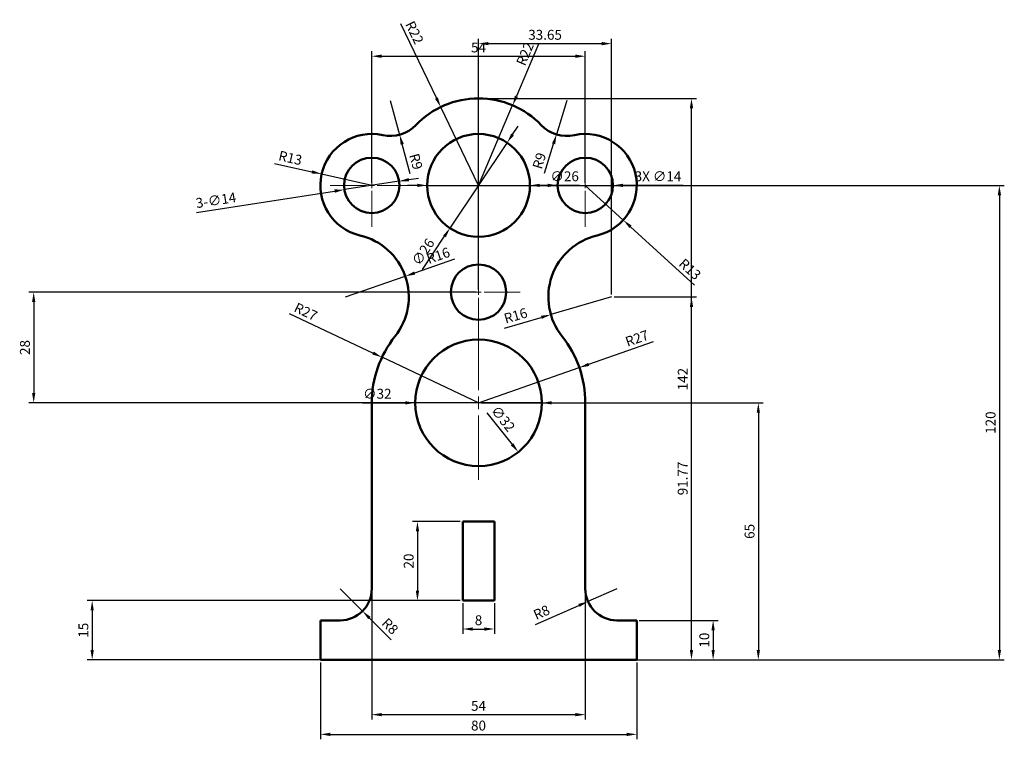
# Model space of a CAD drawing. Units: millimetres. Extents: x 2632 to 2881, y 1283 to 1465.
import ezdxf

# ---------------------------------------------------------------- set-up
doc = ezdxf.new("R2010")
doc.units = ezdxf.units.MM
doc.linetypes.add('CENTER', pattern=[50.8, 31.75, -6.35, 6.35, -6.35])
for name, color, linetype, lineweight in [('M-CNTR', 1, 'CENTER', 18), ('M-DIMS', 2, 'Continuous', 25), ('M-OUTL', 7, 'Continuous', 50)]:
    doc.layers.add(name, color=color, linetype=linetype, lineweight=lineweight)
doc.styles.get("Standard").update_dxf_attribs({"font": 'arial.ttf'})
doc.dimstyles.new('ISO-25', dxfattribs={"dimtxt": 2.5, "dimasz": 2.5, "dimexe": 1.25, "dimexo": 0.625, "dimtad": 1, "dimtxsty": 'Standard', "dimcen": 2.5, "dimadec": 0, "dimazin": 0, "dimtfac": 1, "dimtmove": 0, "dimatfit": 3, "dimfxl": 1, "dimarcsym": 0})

# ---------------------------------------------------------------- blocks, each defined once
blk = doc.blocks.new('*D1')
at = {"layer": 'Defpoints', "color": 0, "transparency": 16777216}
for p in [(2725.72, 1444.66), (2728.09, 1435.98)]:
    blk.add_point(p, dxfattribs=at)
at = {"layer": 'M-DIMS', "color": 0, "lineweight": -2, "transparency": 16777216}
for p, q in [((2725.72, 1444.66), (2728.09, 1435.98)), ((2730.79, 1426.06), (2728.74, 1433.57))]:
    blk.add_line(p, q, dxfattribs=at)
at = {"layer": 'M-DIMS', "color": 0, "transparency": 16777216}
blk.add_solid([(2729.15, 1433.68), (2728.34, 1433.46), (2728.09, 1435.98)], dxfattribs=at)
at = {"layer": 'M-DIMS', "color": 0, "transparency": 16777216, "insert": (2731.93, 1429.11), "char_height": 2.5, "attachment_point": 5, "rotation": 285.2542}
blk.add_mtext('R9', dxfattribs=at)
blk = doc.blocks.new('*D2')
at = {"layer": 'Defpoints', "color": 0, "transparency": 16777216}
for p in [(2738.49, 1442.98), (2748.05, 1423.16)]:
    blk.add_point(p, dxfattribs=at)
at = {"layer": 'M-DIMS', "color": 0, "lineweight": -2, "transparency": 16777216}
for p, q in [((2728.31, 1464.1), (2737.41, 1445.23)), ((2748.05, 1423.16), (2738.49, 1442.98))]:
    blk.add_line(p, q, dxfattribs=at)
at = {"layer": 'M-DIMS', "color": 0, "transparency": 16777216}
blk.add_solid([(2737.78, 1445.41), (2737.03, 1445.05), (2738.49, 1442.98)], dxfattribs=at)
at = {"layer": 'M-DIMS', "color": 0, "transparency": 16777216, "insert": (2731.57, 1461.67), "char_height": 2.5, "attachment_point": 5, "rotation": 295.7492}
blk.add_mtext('R22', dxfattribs=at)
blk = doc.blocks.new('*D3')
at = {"layer": 'Defpoints', "color": 0, "transparency": 16777216}
for p in [(2723.64, 1379.69), (2748.05, 1368.16)]:
    blk.add_point(p, dxfattribs=at)
at = {"layer": 'M-DIMS', "color": 0, "lineweight": -2, "transparency": 16777216}
for p, q in [((2700.16, 1390.77), (2721.38, 1380.76)), ((2748.05, 1368.16), (2723.64, 1379.69))]:
    blk.add_line(p, q, dxfattribs=at)
at = {"layer": 'M-DIMS', "color": 0, "transparency": 16777216}
blk.add_solid([(2721.55, 1381.13), (2721.2, 1380.38), (2723.64, 1379.69)], dxfattribs=at)
at = {"layer": 'M-DIMS', "color": 0, "transparency": 16777216, "insert": (2704.23, 1390.93), "char_height": 2.5, "attachment_point": 5, "rotation": 334.7293}
blk.add_mtext('R27', dxfattribs=at)
blk = doc.blocks.new('*D4')
at = {"layer": 'Defpoints', "color": 0, "transparency": 16777216}
for p in [(2781.7, 1394.94), (2766.33, 1390.48)]:
    blk.add_point(p, dxfattribs=at)
at = {"layer": 'M-DIMS', "color": 0, "lineweight": -2, "transparency": 16777216}
for p, q in [((2781.7, 1394.94), (2766.33, 1390.48)), ((2754.59, 1387.08), (2763.93, 1389.79))]:
    blk.add_line(p, q, dxfattribs=at)
at = {"layer": 'M-DIMS', "color": 0, "transparency": 16777216}
blk.add_solid([(2763.82, 1390.19), (2764.05, 1389.39), (2766.33, 1390.48)], dxfattribs=at)
at = {"layer": 'M-DIMS', "color": 0, "transparency": 16777216, "insert": (2757.53, 1389.92), "char_height": 2.5, "attachment_point": 5, "rotation": 16.1542}
blk.add_mtext('R16', dxfattribs=at)
blk = doc.blocks.new('*D5')
at = {"layer": 'Defpoints', "color": 0, "transparency": 16777216}
for p in [(2783.05, 1321.16), (2775.73, 1317.94)]:
    blk.add_point(p, dxfattribs=at)
at = {"layer": 'M-DIMS', "color": 0, "lineweight": -2, "transparency": 16777216}
for p, q in [((2783.05, 1321.16), (2775.73, 1317.94)), ((2762.45, 1312.1), (2773.44, 1316.93))]:
    blk.add_line(p, q, dxfattribs=at)
at = {"layer": 'M-DIMS', "color": 0, "transparency": 16777216}
blk.add_solid([(2773.27, 1317.32), (2773.61, 1316.55), (2775.73, 1317.94)], dxfattribs=at)
at = {"layer": 'M-DIMS', "color": 0, "transparency": 16777216, "insert": (2764.11, 1314.9), "char_height": 2.5, "attachment_point": 5, "rotation": 23.7502}
blk.add_mtext('R8', dxfattribs=at)
blk = doc.blocks.new('*D6')
at = {"layer": 'Defpoints', "color": 0, "transparency": 16777216}
for p in [(2737.99, 1380.6), (2758.12, 1355.73)]:
    blk.add_point(p, dxfattribs=at)
at = {"layer": 'M-DIMS', "color": 0, "lineweight": -2, "transparency": 16777216}
blk.add_line((2750.11, 1365.62), (2756.54, 1357.67), dxfattribs=at)
blk.add_arc((2748.05, 1368.16), 16, 272.2381, 313.4564, dxfattribs=at)
at = {"layer": 'M-DIMS', "color": 0, "transparency": 16777216}
blk.add_solid([(2756.87, 1357.93), (2756.22, 1357.41), (2758.12, 1355.73)], dxfattribs=at)
at = {"layer": 'M-DIMS', "color": 0, "transparency": 16777216, "insert": (2754.01, 1363.94), "char_height": 2.5, "attachment_point": 5, "rotation": 308.9801}
blk.add_mtext('∅32', dxfattribs=at)
blk = doc.blocks.new('*D7')
at = {"layer": 'Defpoints', "color": 0, "transparency": 16777216}
for p in [(2755.28, 1433.97), (2740.83, 1412.36)]:
    blk.add_point(p, dxfattribs=at)
at = {"layer": 'M-DIMS', "color": 0, "lineweight": -2, "transparency": 16777216}
for p, q in [((2756.67, 1436.05), (2758.06, 1438.13)), ((2755.28, 1433.97), (2740.83, 1412.36)), ((2733.85, 1401.92), (2739.44, 1410.28))]:
    blk.add_line(p, q, dxfattribs=at)
blk.add_arc((2748.05, 1423.16), 13, 230.7308, 267.2454, dxfattribs=at)
at = {"layer": 'M-DIMS', "color": 0, "transparency": 16777216}
for points in [[(2756.32, 1436.28), (2757.01, 1435.82), (2755.28, 1433.97)], [(2739.09, 1410.51), (2739.79, 1410.05), (2740.83, 1412.36)]]:
    blk.add_solid(points, dxfattribs=at)
at = {"layer": 'M-DIMS', "color": 0, "transparency": 16777216, "insert": (2734.31, 1406.16), "char_height": 2.5, "attachment_point": 5, "rotation": 56.24}
blk.add_mtext('∅26', dxfattribs=at)
blk = doc.blocks.new('*D8')
at = {"layer": 'Defpoints', "color": 0, "transparency": 16777216}
for p in [(2714.13, 1422.1), (2727.97, 1424.23)]:
    blk.add_point(p, dxfattribs=at)
at = {"layer": 'M-DIMS', "color": 0, "lineweight": -2, "transparency": 16777216}
for p, q in [((2730.44, 1424.61), (2732.91, 1424.99)), ((2727.97, 1424.23), (2714.13, 1422.1)), ((2676.74, 1416.33), (2711.66, 1421.71))]:
    blk.add_line(p, q, dxfattribs=at)
at = {"layer": 'M-DIMS', "color": 0, "transparency": 16777216}
for points in [[(2730.38, 1425.02), (2730.5, 1424.2), (2727.97, 1424.23)], [(2711.6, 1422.13), (2711.73, 1421.3), (2714.13, 1422.1)]]:
    blk.add_solid(points, dxfattribs=at)
at = {"layer": 'M-DIMS', "color": 0, "transparency": 16777216, "insert": (2681.7, 1419.09), "char_height": 2.5, "attachment_point": 5, "rotation": 8.7711}
blk.add_mtext('3-∅14', dxfattribs=at)
blk = doc.blocks.new('*D9')
at = {"layer": 'Defpoints', "color": 0, "transparency": 16777216}
for p in [(2708.05, 1303.16), (2788.05, 1303.16), (2788.05, 1284.33)]:
    blk.add_point(p, dxfattribs=at)
at = {"layer": 'M-DIMS', "color": 0, "lineweight": -2, "transparency": 16777216}
for p, q in [((2708.05, 1302.54), (2708.05, 1283.08)), ((2788.05, 1302.54), (2788.05, 1283.08)), ((2710.55, 1284.33), (2785.55, 1284.33))]:
    blk.add_line(p, q, dxfattribs=at)
at = {"layer": 'M-DIMS', "color": 0, "transparency": 16777216}
for points in [[(2710.55, 1284.74), (2710.55, 1283.91), (2708.05, 1284.33)], [(2785.55, 1284.74), (2785.55, 1283.91), (2788.05, 1284.33)]]:
    blk.add_solid(points, dxfattribs=at)
at = {"layer": 'M-DIMS', "color": 0, "transparency": 16777216, "insert": (2748.05, 1286.23), "char_height": 2.5, "attachment_point": 5}
blk.add_mtext('80', dxfattribs=at)
blk = doc.blocks.new('*D10')
at = {"layer": 'Defpoints', "color": 0, "transparency": 16777216}
for p in [(2748.05, 1368.16), (2748.05, 1303.16), (2818.81, 1303.16)]:
    blk.add_point(p, dxfattribs=at)
at = {"layer": 'M-DIMS', "color": 0, "lineweight": -2, "transparency": 16777216}
for p, q in [((2748.68, 1368.16), (2820.06, 1368.16)), ((2818.81, 1365.66), (2818.81, 1305.66)), ((2748.68, 1303.16), (2820.06, 1303.16))]:
    blk.add_line(p, q, dxfattribs=at)
at = {"layer": 'M-DIMS', "color": 0, "transparency": 16777216}
for points in [[(2818.39, 1365.66), (2819.22, 1365.66), (2818.81, 1368.16)], [(2818.39, 1305.66), (2819.22, 1305.66), (2818.81, 1303.16)]]:
    blk.add_solid(points, dxfattribs=at)
at = {"layer": 'M-DIMS', "color": 0, "transparency": 16777216, "insert": (2816.91, 1335.66), "char_height": 2.5, "attachment_point": 5, "rotation": 90}
blk.add_mtext('65', dxfattribs=at)
blk = doc.blocks.new('*D11')
at = {"layer": 'Defpoints', "color": 0, "transparency": 16777216}
for p in [(2748.05, 1423.16), (2748.05, 1303.16), (2879.76, 1303.16)]:
    blk.add_point(p, dxfattribs=at)
at = {"layer": 'M-DIMS', "color": 0, "lineweight": -2, "transparency": 16777216}
for p, q in [((2748.68, 1423.16), (2881.01, 1423.16)), ((2879.76, 1420.66), (2879.76, 1305.66)), ((2748.68, 1303.16), (2881.01, 1303.16))]:
    blk.add_line(p, q, dxfattribs=at)
at = {"layer": 'M-DIMS', "color": 0, "transparency": 16777216}
for points in [[(2879.34, 1420.66), (2880.18, 1420.66), (2879.76, 1423.16)], [(2879.34, 1305.66), (2880.18, 1305.66), (2879.76, 1303.16)]]:
    blk.add_solid(points, dxfattribs=at)
at = {"layer": 'M-DIMS', "color": 0, "transparency": 16777216, "insert": (2877.86, 1363.16), "char_height": 2.5, "attachment_point": 5, "rotation": 90}
blk.add_mtext('120', dxfattribs=at)
blk = doc.blocks.new('*D12')
at = {"layer": 'Defpoints', "color": 0, "transparency": 16777216}
for p in [(2788.05, 1313.16), (2788.05, 1303.16), (2807.37, 1303.16)]:
    blk.add_point(p, dxfattribs=at)
at = {"layer": 'M-DIMS', "color": 0, "lineweight": -2, "transparency": 16777216}
for p, q in [((2788.68, 1313.16), (2808.62, 1313.16)), ((2807.37, 1310.66), (2807.37, 1305.66)), ((2788.68, 1303.16), (2808.62, 1303.16))]:
    blk.add_line(p, q, dxfattribs=at)
at = {"layer": 'M-DIMS', "color": 0, "transparency": 16777216}
for points in [[(2806.96, 1310.66), (2807.79, 1310.66), (2807.37, 1313.16)], [(2806.96, 1305.66), (2807.79, 1305.66), (2807.37, 1303.16)]]:
    blk.add_solid(points, dxfattribs=at)
at = {"layer": 'M-DIMS', "color": 0, "transparency": 16777216, "insert": (2805.47, 1308.16), "char_height": 2.5, "attachment_point": 5, "rotation": 90}
blk.add_mtext('10', dxfattribs=at)
blk = doc.blocks.new('*D13')
at = {"layer": 'Defpoints', "color": 0, "transparency": 16777216}
for p in [(2748.05, 1396.16), (2635.56, 1368.16), (2748.05, 1368.16)]:
    blk.add_point(p, dxfattribs=at)
at = {"layer": 'M-DIMS', "color": 0, "lineweight": -2, "transparency": 16777216}
for p, q in [((2747.43, 1396.16), (2634.31, 1396.16)), ((2635.56, 1393.66), (2635.56, 1370.66)), ((2747.43, 1368.16), (2634.31, 1368.16))]:
    blk.add_line(p, q, dxfattribs=at)
at = {"layer": 'M-DIMS', "color": 0, "transparency": 16777216}
for points in [[(2635.14, 1393.66), (2635.98, 1393.66), (2635.56, 1396.16)], [(2635.14, 1370.66), (2635.98, 1370.66), (2635.56, 1368.16)]]:
    blk.add_solid(points, dxfattribs=at)
at = {"layer": 'M-DIMS', "color": 0, "transparency": 16777216, "insert": (2633.66, 1382.16), "char_height": 2.5, "attachment_point": 5, "rotation": 90}
blk.add_mtext('28', dxfattribs=at)
blk = doc.blocks.new('*D14')
at = {"layer": 'Defpoints', "color": 0, "transparency": 16777216}
for p in [(2744.05, 1318.16), (2650.35, 1303.16), (2744.05, 1303.16)]:
    blk.add_point(p, dxfattribs=at)
at = {"layer": 'M-DIMS', "color": 0, "lineweight": -2, "transparency": 16777216}
for p, q in [((2743.43, 1318.16), (2649.1, 1318.16)), ((2650.35, 1315.66), (2650.35, 1305.66)), ((2743.43, 1303.16), (2649.1, 1303.16))]:
    blk.add_line(p, q, dxfattribs=at)
at = {"layer": 'M-DIMS', "color": 0, "transparency": 16777216}
for points in [[(2649.93, 1315.66), (2650.76, 1315.66), (2650.35, 1318.16)], [(2649.93, 1305.66), (2650.76, 1305.66), (2650.35, 1303.16)]]:
    blk.add_solid(points, dxfattribs=at)
at = {"layer": 'M-DIMS', "color": 0, "transparency": 16777216, "insert": (2648.45, 1310.66), "char_height": 2.5, "attachment_point": 5, "rotation": 90}
blk.add_mtext('15', dxfattribs=at)
blk = doc.blocks.new('*D15')
at = {"layer": 'Defpoints', "color": 0, "transparency": 16777216}
for p in [(2775.05, 1455.83), (2721.05, 1423.16), (2775.05, 1423.16)]:
    blk.add_point(p, dxfattribs=at)
at = {"layer": 'M-DIMS', "color": 0, "lineweight": -2, "transparency": 16777216}
for p, q in [((2721.05, 1423.79), (2721.05, 1457.08)), ((2775.05, 1423.79), (2775.05, 1457.08)), ((2723.55, 1455.83), (2772.55, 1455.83))]:
    blk.add_line(p, q, dxfattribs=at)
at = {"layer": 'M-DIMS', "color": 0, "transparency": 16777216}
for points in [[(2723.55, 1456.24), (2723.55, 1455.41), (2721.05, 1455.83)], [(2772.55, 1456.24), (2772.55, 1455.41), (2775.05, 1455.83)]]:
    blk.add_solid(points, dxfattribs=at)
at = {"layer": 'M-DIMS', "color": 0, "transparency": 16777216, "insert": (2748.05, 1457.72), "char_height": 2.5, "attachment_point": 5}
blk.add_mtext('54', dxfattribs=at)
blk = doc.blocks.new('*D16')
at = {"layer": 'Defpoints', "color": 0, "transparency": 16777216}
for p in [(2744.05, 1318.16), (2752.05, 1318.16), (2752.05, 1310.97)]:
    blk.add_point(p, dxfattribs=at)
at = {"layer": 'M-DIMS', "color": 0, "lineweight": -2, "transparency": 16777216}
for p, q in [((2744.05, 1317.54), (2744.05, 1309.72)), ((2752.05, 1317.54), (2752.05, 1309.72)), ((2746.55, 1310.97), (2749.55, 1310.97))]:
    blk.add_line(p, q, dxfattribs=at)
at = {"layer": 'M-DIMS', "color": 0, "transparency": 16777216}
for points in [[(2746.55, 1311.38), (2746.55, 1310.55), (2744.05, 1310.97)], [(2749.55, 1311.38), (2749.55, 1310.55), (2752.05, 1310.97)]]:
    blk.add_solid(points, dxfattribs=at)
at = {"layer": 'M-DIMS', "color": 0, "transparency": 16777216, "insert": (2748.05, 1312.87), "char_height": 2.5, "attachment_point": 5}
blk.add_mtext('8', dxfattribs=at)
blk = doc.blocks.new('*D17')
at = {"layer": 'Defpoints', "color": 0, "transparency": 16777216}
for p in [(2775.05, 1423.16), (2784.65, 1414.39)]:
    blk.add_point(p, dxfattribs=at)
at = {"layer": 'M-DIMS', "color": 0, "lineweight": -2, "transparency": 16777216}
for p, q in [((2775.05, 1423.16), (2784.65, 1414.39)), ((2802.69, 1397.9), (2786.49, 1412.71))]:
    blk.add_line(p, q, dxfattribs=at)
at = {"layer": 'M-DIMS', "color": 0, "transparency": 16777216}
blk.add_solid([(2786.77, 1413.01), (2786.21, 1412.4), (2784.65, 1414.39)], dxfattribs=at)
at = {"layer": 'M-DIMS', "color": 0, "transparency": 16777216, "insert": (2801.3, 1401.74), "char_height": 2.5, "attachment_point": 5, "rotation": 317.5657}
blk.add_mtext('R13', dxfattribs=at)
blk = doc.blocks.new('*D18')
at = {"layer": 'Defpoints', "color": 0, "transparency": 16777216}
for p in [(2744.05, 1338.16), (2732.6, 1318.16), (2744.05, 1318.16)]:
    blk.add_point(p, dxfattribs=at)
at = {"layer": 'M-DIMS', "color": 0, "lineweight": -2, "transparency": 16777216}
for p, q in [((2743.43, 1338.16), (2731.35, 1338.16)), ((2732.6, 1335.66), (2732.6, 1320.66)), ((2743.43, 1318.16), (2731.35, 1318.16))]:
    blk.add_line(p, q, dxfattribs=at)
at = {"layer": 'M-DIMS', "color": 0, "transparency": 16777216}
for points in [[(2732.19, 1335.66), (2733.02, 1335.66), (2732.6, 1338.16)], [(2732.19, 1320.66), (2733.02, 1320.66), (2732.6, 1318.16)]]:
    blk.add_solid(points, dxfattribs=at)
at = {"layer": 'M-DIMS', "color": 0, "transparency": 16777216, "insert": (2730.7, 1328.16), "char_height": 2.5, "attachment_point": 5, "rotation": 90}
blk.add_mtext('20', dxfattribs=at)
blk = doc.blocks.new('*U19')
at = {"layer": 'M-CNTR', "color": 0, "transparency": 16777216}
for p, q in [((0, 2.6), (0, 16.5)), ((-16.5, 0), (-2.6, 0)), ((2.6, 0), (16.5, 0)), ((0, -16.5), (0, -2.6))]:
    blk.add_line(p, q, dxfattribs=at)
at = {"layer": 'M-CNTR', "color": 0, "linetype": 'Continuous', "transparency": 16777216}
for p, q in [((-1.3, 0), (1.3, 0)), ((0, -1.3), (0, 1.3))]:
    blk.add_line(p, q, dxfattribs=at)
blk = doc.blocks.new('*U20')
at = {"layer": 'M-CNTR', "color": 0, "transparency": 16777216}
for p, q in [((0, 3.2), (0, 19.5)), ((-19.5, 0), (-3.2, 0)), ((3.2, 0), (19.5, 0)), ((0, -19.5), (0, -3.2))]:
    blk.add_line(p, q, dxfattribs=at)
at = {"layer": 'M-CNTR', "color": 0, "linetype": 'Continuous', "transparency": 16777216}
for p, q in [((-1.6, 0), (1.6, 0)), ((0, -1.6), (0, 1.6))]:
    blk.add_line(p, q, dxfattribs=at)
blk = doc.blocks.new('*U21')
at = {"layer": 'M-CNTR', "color": 0, "transparency": 16777216}
for p, q in [((0, 3.2), (0, 19.5)), ((-19.5, 0), (-3.2, 0)), ((3.2, 0), (19.5, 0)), ((0, -19.5), (0, -3.2))]:
    blk.add_line(p, q, dxfattribs=at)
at = {"layer": 'M-CNTR', "color": 0, "linetype": 'Continuous', "transparency": 16777216}
for p, q in [((-1.6, 0), (1.6, 0)), ((0, -1.6), (0, 1.6))]:
    blk.add_line(p, q, dxfattribs=at)
blk = doc.blocks.new('*U22')
at = {"layer": 'M-CNTR', "color": 0, "transparency": 16777216}
for p, q in [((0, 1.4), (0, 10.5)), ((-10.5, 0), (-1.4, 0)), ((1.4, 0), (10.5, 0)), ((0, -10.5), (0, -1.4))]:
    blk.add_line(p, q, dxfattribs=at)
at = {"layer": 'M-CNTR', "color": 0, "linetype": 'Continuous', "transparency": 16777216}
for p, q in [((-0.7, 0), (0.7, 0)), ((0, -0.7), (0, 0.7))]:
    blk.add_line(p, q, dxfattribs=at)
blk = doc.blocks.new('*U23')
at = {"layer": 'M-CNTR', "color": 0, "transparency": 16777216}
for p, q in [((0, 1.4), (0, 10.5)), ((-10.5, 0), (-1.4, 0)), ((1.4, 0), (10.5, 0)), ((0, -10.5), (0, -1.4))]:
    blk.add_line(p, q, dxfattribs=at)
at = {"layer": 'M-CNTR', "color": 0, "linetype": 'Continuous', "transparency": 16777216}
for p, q in [((-0.7, 0), (0.7, 0)), ((0, -0.7), (0, 0.7))]:
    blk.add_line(p, q, dxfattribs=at)
blk = doc.blocks.new('*U24')
at = {"layer": 'M-CNTR', "color": 0, "transparency": 16777216}
for p, q in [((0, 1.4), (0, 10.5)), ((-10.5, 0), (-1.4, 0)), ((1.4, 0), (10.5, 0)), ((0, -10.5), (0, -1.4))]:
    blk.add_line(p, q, dxfattribs=at)
at = {"layer": 'M-CNTR', "color": 0, "linetype": 'Continuous', "transparency": 16777216}
for p, q in [((-0.7, 0), (0.7, 0)), ((0, -0.7), (0, 0.7))]:
    blk.add_line(p, q, dxfattribs=at)
blk = doc.blocks.new('*U25')
at = {"layer": 'M-CNTR', "color": 0, "transparency": 16777216}
for p, q in [((0, 1.4), (0, 10.5)), ((-10.5, 0), (-1.4, 0)), ((1.4, 0), (10.5, 0)), ((0, -10.5), (0, -1.4))]:
    blk.add_line(p, q, dxfattribs=at)
at = {"layer": 'M-CNTR', "color": 0, "linetype": 'Continuous', "transparency": 16777216}
for p, q in [((-0.7, 0), (0.7, 0)), ((0, -0.7), (0, 0.7))]:
    blk.add_line(p, q, dxfattribs=at)
blk = doc.blocks.new('*D26')
at = {"layer": 'Defpoints', "color": 0, "transparency": 16777216}
for p in [(2721.05, 1368.16), (2775.05, 1368.16), (2775.05, 1289.31)]:
    blk.add_point(p, dxfattribs=at)
at = {"layer": 'M-DIMS', "color": 0, "lineweight": -2, "transparency": 16777216}
for p, q in [((2721.05, 1367.54), (2721.05, 1288.06)), ((2775.05, 1367.54), (2775.05, 1288.06)), ((2723.55, 1289.31), (2772.55, 1289.31))]:
    blk.add_line(p, q, dxfattribs=at)
at = {"layer": 'M-DIMS', "color": 0, "transparency": 16777216}
for points in [[(2723.55, 1289.73), (2723.55, 1288.9), (2721.05, 1289.31)], [(2772.55, 1289.73), (2772.55, 1288.9), (2775.05, 1289.31)]]:
    blk.add_solid(points, dxfattribs=at)
at = {"layer": 'M-DIMS', "color": 0, "transparency": 16777216, "insert": (2748.05, 1291.21), "char_height": 2.5, "attachment_point": 5}
blk.add_mtext('54', dxfattribs=at)
blk = doc.blocks.new('*D27')
at = {"layer": 'Defpoints', "color": 0, "transparency": 16777216}
for p in [(2781.7, 1459.01), (2748.05, 1396.16), (2781.7, 1394.94)]:
    blk.add_point(p, dxfattribs=at)
at = {"layer": 'M-DIMS', "color": 0, "lineweight": -2, "transparency": 16777216}
for p, q in [((2748.05, 1396.79), (2748.05, 1460.26)), ((2781.7, 1395.56), (2781.7, 1460.26)), ((2750.55, 1459.01), (2779.2, 1459.01))]:
    blk.add_line(p, q, dxfattribs=at)
at = {"layer": 'M-DIMS', "color": 0, "transparency": 16777216}
for points in [[(2750.55, 1459.43), (2750.55, 1458.6), (2748.05, 1459.01)], [(2779.2, 1459.43), (2779.2, 1458.6), (2781.7, 1459.01)]]:
    blk.add_solid(points, dxfattribs=at)
at = {"layer": 'M-DIMS', "color": 0, "transparency": 16777216, "insert": (2764.88, 1460.92), "char_height": 2.5, "attachment_point": 5}
blk.add_mtext('33.65', dxfattribs=at)
blk = doc.blocks.new('*D28')
at = {"layer": 'Defpoints', "color": 0, "transparency": 16777216}
for p in [(2781.7, 1394.94), (2801.9, 1394.94), (2788.05, 1303.16)]:
    blk.add_point(p, dxfattribs=at)
at = {"layer": 'M-DIMS', "color": 0, "lineweight": -2, "transparency": 16777216}
for p, q in [((2782.33, 1394.94), (2803.15, 1394.94)), ((2801.9, 1305.66), (2801.9, 1392.44)), ((2788.68, 1303.16), (2803.15, 1303.16))]:
    blk.add_line(p, q, dxfattribs=at)
at = {"layer": 'M-DIMS', "color": 0, "transparency": 16777216}
for points in [[(2801.49, 1392.44), (2802.32, 1392.44), (2801.9, 1394.94)], [(2801.49, 1305.66), (2802.32, 1305.66), (2801.9, 1303.16)]]:
    blk.add_solid(points, dxfattribs=at)
at = {"layer": 'M-DIMS', "color": 0, "transparency": 16777216, "insert": (2800, 1349.05), "char_height": 2.5, "attachment_point": 5, "rotation": 90}
blk.add_mtext('91.77', dxfattribs=at)
blk = doc.blocks.new('*D29')
at = {"layer": 'Defpoints', "color": 0, "transparency": 16777216}
for p in [(2748.05, 1445.16), (2801.9, 1445.16), (2788.05, 1303.16)]:
    blk.add_point(p, dxfattribs=at)
at = {"layer": 'M-DIMS', "color": 0, "lineweight": -2, "transparency": 16777216}
for p, q in [((2748.68, 1445.16), (2803.15, 1445.16)), ((2801.9, 1305.66), (2801.9, 1442.66)), ((2788.68, 1303.16), (2803.15, 1303.16))]:
    blk.add_line(p, q, dxfattribs=at)
at = {"layer": 'M-DIMS', "color": 0, "transparency": 16777216}
for points in [[(2801.49, 1442.66), (2802.32, 1442.66), (2801.9, 1445.16)], [(2801.49, 1305.66), (2802.32, 1305.66), (2801.9, 1303.16)]]:
    blk.add_solid(points, dxfattribs=at)
at = {"layer": 'M-DIMS', "color": 0, "transparency": 16777216, "insert": (2800.02, 1374.16), "char_height": 2.5, "attachment_point": 5, "rotation": 90}
blk.add_mtext('142', dxfattribs=at)
blk = doc.blocks.new('*D30')
at = {"layer": 'Defpoints', "color": 0, "transparency": 16777216}
for p in [(2732.05, 1368.16), (2764.05, 1368.16)]:
    blk.add_point(p, dxfattribs=at)
at = {"layer": 'M-DIMS', "color": 0, "lineweight": -2, "transparency": 16777216}
for p, q in [((2718.69, 1368.16), (2729.55, 1368.16)), ((2764.05, 1368.16), (2732.05, 1368.16)), ((2766.55, 1368.16), (2769.05, 1368.16))]:
    blk.add_line(p, q, dxfattribs=at)
at = {"layer": 'M-DIMS', "color": 0, "transparency": 16777216}
for points in [[(2729.55, 1368.58), (2729.55, 1367.75), (2732.05, 1368.16)], [(2766.55, 1368.58), (2766.55, 1367.75), (2764.05, 1368.16)]]:
    blk.add_solid(points, dxfattribs=at)
at = {"layer": 'M-DIMS', "color": 0, "transparency": 16777216, "insert": (2722.45, 1370.14), "char_height": 2.5, "attachment_point": 5, "rotation": 359.9986}
blk.add_mtext('∅32', dxfattribs=at)
blk = doc.blocks.new('*D31')
at = {"layer": 'Defpoints', "color": 0, "transparency": 16777216}
for p in [(2735.05, 1423.16), (2761.05, 1423.16)]:
    blk.add_point(p, dxfattribs=at)
at = {"layer": 'M-DIMS', "color": 0, "lineweight": -2, "transparency": 16777216}
for p, q in [((2732.55, 1423.16), (2730.05, 1423.16)), ((2735.05, 1423.16), (2761.05, 1423.16)), ((2773.6, 1423.16), (2763.55, 1423.16))]:
    blk.add_line(p, q, dxfattribs=at)
at = {"layer": 'M-DIMS', "color": 0, "transparency": 16777216}
for points in [[(2732.55, 1423.58), (2732.55, 1422.75), (2735.05, 1423.16)], [(2763.55, 1423.58), (2763.55, 1422.75), (2761.05, 1423.16)]]:
    blk.add_solid(points, dxfattribs=at)
at = {"layer": 'M-DIMS', "color": 0, "transparency": 16777216, "insert": (2769.83, 1425.14), "char_height": 2.5, "attachment_point": 5, "rotation": 0.0017}
blk.add_mtext('∅26', dxfattribs=at)
blk = doc.blocks.new('*D32')
at = {"layer": 'Defpoints', "color": 0, "transparency": 16777216}
for p in [(2768.05, 1423.16), (2782.05, 1423.16)]:
    blk.add_point(p, dxfattribs=at)
at = {"layer": 'M-DIMS', "color": 0, "lineweight": -2, "transparency": 16777216}
for p, q in [((2765.55, 1423.16), (2763.05, 1423.16)), ((2768.05, 1423.16), (2782.05, 1423.16)), ((2799.83, 1423.16), (2784.55, 1423.16))]:
    blk.add_line(p, q, dxfattribs=at)
at = {"layer": 'M-DIMS', "color": 0, "transparency": 16777216}
for points in [[(2765.55, 1423.58), (2765.55, 1422.75), (2768.05, 1423.16)], [(2784.55, 1423.58), (2784.55, 1422.75), (2782.05, 1423.16)]]:
    blk.add_solid(points, dxfattribs=at)
at = {"layer": 'M-DIMS', "color": 0, "transparency": 16777216, "insert": (2793.44, 1425.14), "char_height": 2.5, "attachment_point": 5, "rotation": 0.0031}
blk.add_mtext('3X ∅14', dxfattribs=at)
blk = doc.blocks.new('*D33')
at = {"layer": 'Defpoints', "color": 0, "transparency": 16777216}
for p in [(2708.37, 1426.03), (2721.05, 1423.16)]:
    blk.add_point(p, dxfattribs=at)
at = {"layer": 'M-DIMS', "color": 0, "lineweight": -2, "transparency": 16777216}
for p, q in [((2696.45, 1428.73), (2705.93, 1426.58)), ((2721.05, 1423.16), (2708.37, 1426.03))]:
    blk.add_line(p, q, dxfattribs=at)
at = {"layer": 'M-DIMS', "color": 0, "transparency": 16777216}
blk.add_solid([(2706.03, 1426.99), (2705.84, 1426.18), (2708.37, 1426.03)], dxfattribs=at)
at = {"layer": 'M-DIMS', "color": 0, "transparency": 16777216, "insert": (2700.39, 1429.79), "char_height": 2.5, "attachment_point": 5, "rotation": 347.2487}
blk.add_mtext('R13', dxfattribs=at)
blk = doc.blocks.new('*D34')
at = {"layer": 'Defpoints', "color": 0, "transparency": 16777216}
for p in [(2773.54, 1377.07), (2748.05, 1368.16)]:
    blk.add_point(p, dxfattribs=at)
at = {"layer": 'M-DIMS', "color": 0, "lineweight": -2, "transparency": 16777216}
for p, q in [((2792.25, 1383.6), (2775.9, 1377.89)), ((2748.05, 1368.16), (2773.54, 1377.07))]:
    blk.add_line(p, q, dxfattribs=at)
at = {"layer": 'M-DIMS', "color": 0, "transparency": 16777216}
blk.add_solid([(2775.77, 1378.28), (2776.04, 1377.5), (2773.54, 1377.07)], dxfattribs=at)
at = {"layer": 'M-DIMS', "color": 0, "transparency": 16777216, "insert": (2788.22, 1384.18), "char_height": 2.5, "attachment_point": 5, "rotation": 19.2541}
blk.add_mtext('R27', dxfattribs=at)
blk = doc.blocks.new('*D35')
at = {"layer": 'Defpoints', "color": 0, "transparency": 16777216}
for p in [(2729.52, 1400.18), (2714.4, 1394.94)]:
    blk.add_point(p, dxfattribs=at)
at = {"layer": 'M-DIMS', "color": 0, "lineweight": -2, "transparency": 16777216}
for p, q in [((2742, 1404.5), (2731.88, 1401)), ((2714.4, 1394.94), (2729.52, 1400.18))]:
    blk.add_line(p, q, dxfattribs=at)
at = {"layer": 'M-DIMS', "color": 0, "transparency": 16777216}
blk.add_solid([(2731.75, 1401.39), (2732.02, 1400.6), (2729.52, 1400.18)], dxfattribs=at)
at = {"layer": 'M-DIMS', "color": 0, "transparency": 16777216, "insert": (2737.97, 1405.12), "char_height": 2.5, "attachment_point": 5, "rotation": 19.1207}
blk.add_mtext('R16', dxfattribs=at)
blk = doc.blocks.new('*D36')
at = {"layer": 'Defpoints', "color": 0, "transparency": 16777216}
for p in [(2756.66, 1443.41), (2748.05, 1423.16)]:
    blk.add_point(p, dxfattribs=at)
at = {"layer": 'M-DIMS', "color": 0, "lineweight": -2, "transparency": 16777216}
for p, q in [((2763.24, 1458.87), (2757.64, 1445.71)), ((2748.05, 1423.16), (2756.66, 1443.41))]:
    blk.add_line(p, q, dxfattribs=at)
at = {"layer": 'M-DIMS', "color": 0, "transparency": 16777216}
blk.add_solid([(2757.26, 1445.87), (2758.03, 1445.55), (2756.66, 1443.41)], dxfattribs=at)
at = {"layer": 'M-DIMS', "color": 0, "transparency": 16777216, "insert": (2760.1, 1456.29), "char_height": 2.5, "attachment_point": 5, "rotation": 66.9562}
blk.add_mtext('R22', dxfattribs=at)
blk = doc.blocks.new('*D37')
at = {"layer": 'Defpoints', "color": 0, "transparency": 16777216}
for p in [(2770.39, 1444.66), (2767.77, 1436.05)]:
    blk.add_point(p, dxfattribs=at)
at = {"layer": 'M-DIMS', "color": 0, "lineweight": -2, "transparency": 16777216}
for p, q in [((2770.39, 1444.66), (2767.77, 1436.05)), ((2764.77, 1426.21), (2767.04, 1433.66))]:
    blk.add_line(p, q, dxfattribs=at)
at = {"layer": 'M-DIMS', "color": 0, "transparency": 16777216}
blk.add_solid([(2766.64, 1433.78), (2767.44, 1433.54), (2767.77, 1436.05)], dxfattribs=at)
at = {"layer": 'M-DIMS', "color": 0, "transparency": 16777216, "insert": (2763.72, 1429.29), "char_height": 2.5, "attachment_point": 5, "rotation": 73.0762}
blk.add_mtext('R9', dxfattribs=at)
blk = doc.blocks.new('*D38')
at = {"layer": 'Defpoints', "color": 0, "transparency": 16777216}
for p in [(2713.05, 1321.16), (2718.71, 1315.51)]:
    blk.add_point(p, dxfattribs=at)
at = {"layer": 'M-DIMS', "color": 0, "lineweight": -2, "transparency": 16777216}
for p, q in [((2713.05, 1321.16), (2718.71, 1315.51)), ((2725.98, 1308.23), (2720.48, 1313.74))]:
    blk.add_line(p, q, dxfattribs=at)
at = {"layer": 'M-DIMS', "color": 0, "transparency": 16777216}
blk.add_solid([(2720.77, 1314.03), (2720.18, 1313.44), (2718.71, 1315.51)], dxfattribs=at)
at = {"layer": 'M-DIMS', "color": 0, "transparency": 16777216, "insert": (2725.46, 1311.45), "char_height": 2.5, "attachment_point": 5, "rotation": 314.9995}
blk.add_mtext('R8', dxfattribs=at)

msp = doc.modelspace()

# ---------------------------------------------------------------- linework, layer by layer
at = {"layer": 'M-OUTL'}
for p, q in [((2721.052, 1321.164), (2721.052, 1368.164)), ((2775.052, 1321.164), (2775.052, 1368.164)), ((2744.052, 1318.164), (2744.052, 1338.164)), ((2744.052, 1318.164), (2744.052, 1338.164)), ((2744.052, 1318.164), (2744.052, 1338.164)), ((2744.052, 1318.164), (2744.052, 1338.164)), ((2744.052, 1318.164), (2744.052, 1338.164)), ((2752.052, 1338.164), (2744.052, 1338.164)), ((2752.052, 1318.164), (2752.052, 1338.164)), ((2752.052, 1318.164), (2744.052, 1318.164)), ((2708.052, 1303.164), (2708.052, 1313.164)), ((2708.052, 1313.164), (2713.052, 1313.164)), ((2788.052, 1313.164), (2783.052, 1313.164)), ((2788.052, 1303.164), (2788.052, 1313.164)), ((2748.052, 1303.164), (2708.052, 1303.164)), ((2748.052, 1303.164), (2788.052, 1303.164))]:
    msp.add_line(p, q, dxfattribs=at)
for centre in [(2721.052, 1423.164), (2775.052, 1423.164)]:
    msp.add_circle(centre, 7, dxfattribs=at)
for centre, radius, start, end in [((2748.052, 1423.164), 22, 90, 136.09), ((2748.052, 1423.164), 22, 43.91, 90), ((2725.719, 1444.663), 9, 257.75331, 316.09), ((2770.386, 1444.663), 9, 223.91, 282.24669), ((2721.052, 1423.164), 13, 77.75331, 256.74614), ((2748.052, 1423.164), 13, 90, 270), ((2748.052, 1423.164), 13, 270, 90), ((2775.052, 1423.164), 13, 283.25386, 102.24669), ((2714.404, 1394.936), 16, 321.49264, 76.74614), ((2781.701, 1394.936), 16, 103.25386, 218.50736), ((2748.052, 1396.164), 7, 90, 270), ((2748.052, 1396.164), 7, 270, 90), ((2748.052, 1368.164), 27, 141.49264, 180), ((2748.052, 1368.164), 27, 0, 38.50736), ((2748.052, 1368.164), 16, 90, 270), ((2748.052, 1368.164), 16, 270, 90), ((2713.052, 1321.164), 8, 270, 0), ((2783.052, 1321.164), 8, 180, 270)]:
    msp.add_arc(centre, radius, start, end, dxfattribs=at)

# ---------------------------------------------------------------- block references
at = {"layer": 'M-CNTR'}
for name, p in [('*U19', (2748.052, 1423.164)), ('*U25', (2721.052, 1423.164)), ('*U24', (2775.052, 1423.164)), ('*U22', (2748.052, 1396.164)), ('*U23', (2748.052, 1396.164)), ('*U20', (2748.052, 1368.164)), ('*U21', (2748.052, 1368.164))]:
    msp.add_blockref(name, p, dxfattribs=at)

# ---------------------------------------------------------------- dimensions: what is measured, and where the dimension line sits
at = {"layer": 'M-DIMS'}
for center, mpoint, override, picture, middle in [((2748.052, 1423.164), (2738.495, 1442.979), {"dimclrd": 0, "dimclre": 0, "dimclrt": 0}, '*D2', (2729.873, 1460.856)), ((2748.052, 1423.164), (2756.664, 1443.408), {"dimdec": 0, "dimlfac": 1, "dimrnd": 0, "dimzin": 0, "dimdsep": 46, "dimlunit": 2}, '*D36', (2761.831, 1455.555)), ((2775.052, 1423.164), (2784.647, 1414.392), {"dimclrd": 0, "dimclre": 0, "dimclrt": 0}, '*D17', (2800.019, 1400.338)), ((2714.404, 1394.936), (2729.521, 1400.177), {"dimdec": 0, "dimlfac": 1, "dimrnd": 0, "dimzin": 0, "dimdsep": 46, "dimlunit": 2}, '*D35', (2738.591, 1403.322)), ((2748.052, 1368.164), (2723.636, 1379.69), {"dimclrd": 0, "dimclre": 0, "dimclrt": 0}, '*D3', (2703.43, 1389.229)), ((2748.052, 1368.164), (2773.542, 1377.067), {"dimdec": 0, "dimlfac": 1, "dimrnd": 0, "dimzin": 0, "dimdsep": 46, "dimlunit": 2}, '*D34', (2788.836, 1382.409)), ((2783.052, 1321.164), (2775.73, 1317.942), {"dimclrd": 0, "dimclre": 0, "dimclrt": 0}, '*D5', (2764.871, 1313.164))]:
    dim = msp.add_radius_dim(center=center, mpoint=mpoint, dimstyle='ISO-25', override=override, dxfattribs=at)
    dim.commit()
    dim.dimension.update_dxf_attribs({"geometry": picture, "text_midpoint": middle, "dimtype": 164})
for base, p1, p2, override, picture, middle in [((2781.701, 1459.014), (2748.052, 1396.164), (2781.701, 1394.936), {"dimdec": 2, "dimlfac": 1, "dimrnd": 0, "dimzin": 0, "dimdsep": 46, "dimlunit": 2}, '*D27', (2764.877, 1460.916)), ((2775.052, 1455.826), (2721.052, 1423.164), (2775.052, 1423.164), {"dimclrd": 0, "dimclre": 0, "dimclrt": 0}, '*D15', (2748.052, 1457.722)), ((2775.052, 1289.314), (2721.052, 1368.164), (2775.052, 1368.164), {"dimdec": 0, "dimlfac": 1, "dimrnd": 0, "dimzin": 0, "dimdsep": 46, "dimlunit": 2}, '*D26', (2748.052, 1291.21)), ((2752.052, 1310.965), (2744.052, 1318.164), (2752.052, 1318.164), {"dimclrd": 0, "dimclre": 0, "dimclrt": 0}, '*D16', (2748.052, 1312.867)), ((2788.052, 1284.327), (2708.052, 1303.164), (2788.052, 1303.164), {"dimclrd": 0, "dimclre": 0, "dimclrt": 0}, '*D9', (2748.052, 1286.229))]:
    dim = msp.add_linear_dim(base=base, p1=p1, p2=p2, dimstyle='ISO-25', override=override, dxfattribs=at)
    dim.commit()
    dim.dimension.update_dxf_attribs({"geometry": picture, "text_midpoint": middle})
for center, mpoint, override, picture, middle in [((2725.719, 1444.663), (2728.087, 1435.98), {"dimclrd": 0, "dimclre": 0, "dimclrt": 0}, '*D1', (2731.932, 1429.106)), ((2770.386, 1444.663), (2767.766, 1436.053), {"dimdec": 0, "dimlfac": 1, "dimrnd": 0, "dimzin": 0, "dimdsep": 46, "dimlunit": 2}, '*D37', (2763.722, 1429.294)), ((2721.052, 1423.164), (2708.373, 1426.033), {"dimdec": 0, "dimlfac": 1, "dimrnd": 0, "dimzin": 0, "dimdsep": 46, "dimlunit": 2}, '*D33', (2700.394, 1429.789)), ((2781.701, 1394.936), (2766.333, 1390.485), {"dimclrd": 0, "dimclre": 0, "dimclrt": 0}, '*D4', (2757.533, 1389.915)), ((2713.052, 1321.164), (2718.709, 1315.507), {"dimdec": 0, "dimlfac": 1, "dimrnd": 0, "dimzin": 0, "dimdsep": 46, "dimlunit": 2}, '*D38', (2725.458, 1311.447))]:
    dim = msp.add_radius_dim(center=center, mpoint=mpoint, dimstyle='ISO-25', override=override, dxfattribs=at)
    dim.commit()
    dim.dimension.update_dxf_attribs({"geometry": picture, "text_midpoint": middle})
for base, p1, p2, override, picture, middle in [((2801.902, 1445.164), (2788.052, 1303.164), (2748.052, 1445.164), {"dimdec": 0, "dimlfac": 1, "dimrnd": 0, "dimzin": 0, "dimdsep": 46, "dimlunit": 2}, '*D29', (2800.022, 1374.164)), ((2879.759, 1303.164), (2748.052, 1423.164), (2748.052, 1303.164), {"dimclrd": 0, "dimclre": 0, "dimclrt": 0}, '*D11', (2877.858, 1363.164)), ((2635.559, 1368.164), (2748.052, 1396.164), (2748.052, 1368.164), {"dimclrd": 0, "dimclre": 0, "dimclrt": 0}, '*D13', (2633.658, 1382.164)), ((2801.902, 1394.936), (2788.052, 1303.164), (2781.701, 1394.936), {"dimdec": 2, "dimlfac": 1, "dimrnd": 0, "dimzin": 0, "dimdsep": 46, "dimlunit": 2}, '*D28', (2800.001, 1349.05)), ((2818.808, 1303.164), (2748.052, 1368.164), (2748.052, 1303.164), {"dimclrd": 0, "dimclre": 0, "dimclrt": 0}, '*D10', (2816.907, 1335.664)), ((2732.603, 1318.164), (2744.052, 1338.164), (2744.052, 1318.164), {"dimclrd": 0, "dimclre": 0, "dimclrt": 0}, '*D18', (2730.702, 1328.164)), ((2650.347, 1303.164), (2744.052, 1318.164), (2744.052, 1303.164), {"dimclrd": 0, "dimclre": 0, "dimclrt": 0}, '*D14', (2648.446, 1310.664)), ((2807.373, 1303.164), (2788.052, 1313.164), (2788.052, 1303.164), {"dimclrd": 0, "dimclre": 0, "dimclrt": 0}, '*D12', (2805.472, 1308.164))]:
    dim = msp.add_linear_dim(base=base, p1=p1, p2=p2, angle=90, dimstyle='ISO-25', override=override, dxfattribs=at)
    dim.commit()
    dim.dimension.update_dxf_attribs({"geometry": picture, "text_midpoint": middle})
for p1, p2, override, picture, middle in [((2755.277, 1433.971), (2740.828, 1412.356), {"dimclrd": 0, "dimclre": 0, "dimclrt": 0}, '*D7', (2734.313, 1406.156)), ((2735.052, 1423.163), (2761.052, 1423.164), {"dimdec": 0, "dimlfac": 1, "dimrnd": 0, "dimzin": 0, "dimdsep": 46, "dimlunit": 2}, '*D31', (2769.827, 1423.164))]:
    dim = msp.add_diameter_dim_2p(p1=p1, p2=p2, dimstyle='ISO-25', override=override, dxfattribs=at)
    dim.commit()
    dim.dimension.update_dxf_attribs({"geometry": picture, "text_midpoint": middle})
dim = msp.add_diameter_dim_2p(p1=(2768.052, 1423.163), p2=(2782.052, 1423.164), text='3X <>', dimstyle='ISO-25', override={"dimdec": 0, "dimlfac": 1, "dimrnd": 0, "dimzin": 0, "dimdsep": 46, "dimlunit": 2}, dxfattribs=at)
dim.commit()
dim.dimension.update_dxf_attribs({"geometry": '*D32', "text_midpoint": (2793.441, 1423.165)})
dim = msp.add_diameter_dim_2p(p1=(2727.971, 1424.231), p2=(2714.134, 1422.096), text='3-<>', dimstyle='ISO-25', override={"dimclrd": 0, "dimclre": 0, "dimclrt": 0}, dxfattribs=at)
dim.commit()
dim.dimension.update_dxf_attribs({"geometry": '*D8', "text_midpoint": (2682, 1417.138), "dimtype": 163})
for p1, p2, override, picture, middle in [((2737.988, 1380.601), (2758.117, 1355.726), {"dimclrd": 0, "dimclre": 0, "dimclrt": 0}, '*D6', (2752.474, 1362.699)), ((2764.052, 1368.163), (2732.052, 1368.164), {"dimdec": 0, "dimlfac": 1, "dimrnd": 0, "dimzin": 0, "dimdsep": 46, "dimlunit": 2}, '*D30', (2722.452, 1368.164))]:
    dim = msp.add_diameter_dim_2p(p1=p1, p2=p2, dimstyle='ISO-25', override=override, dxfattribs=at)
    dim.commit()
    dim.dimension.update_dxf_attribs({"geometry": picture, "text_midpoint": middle, "dimtype": 163})

doc.saveas('drawing.dxf')
